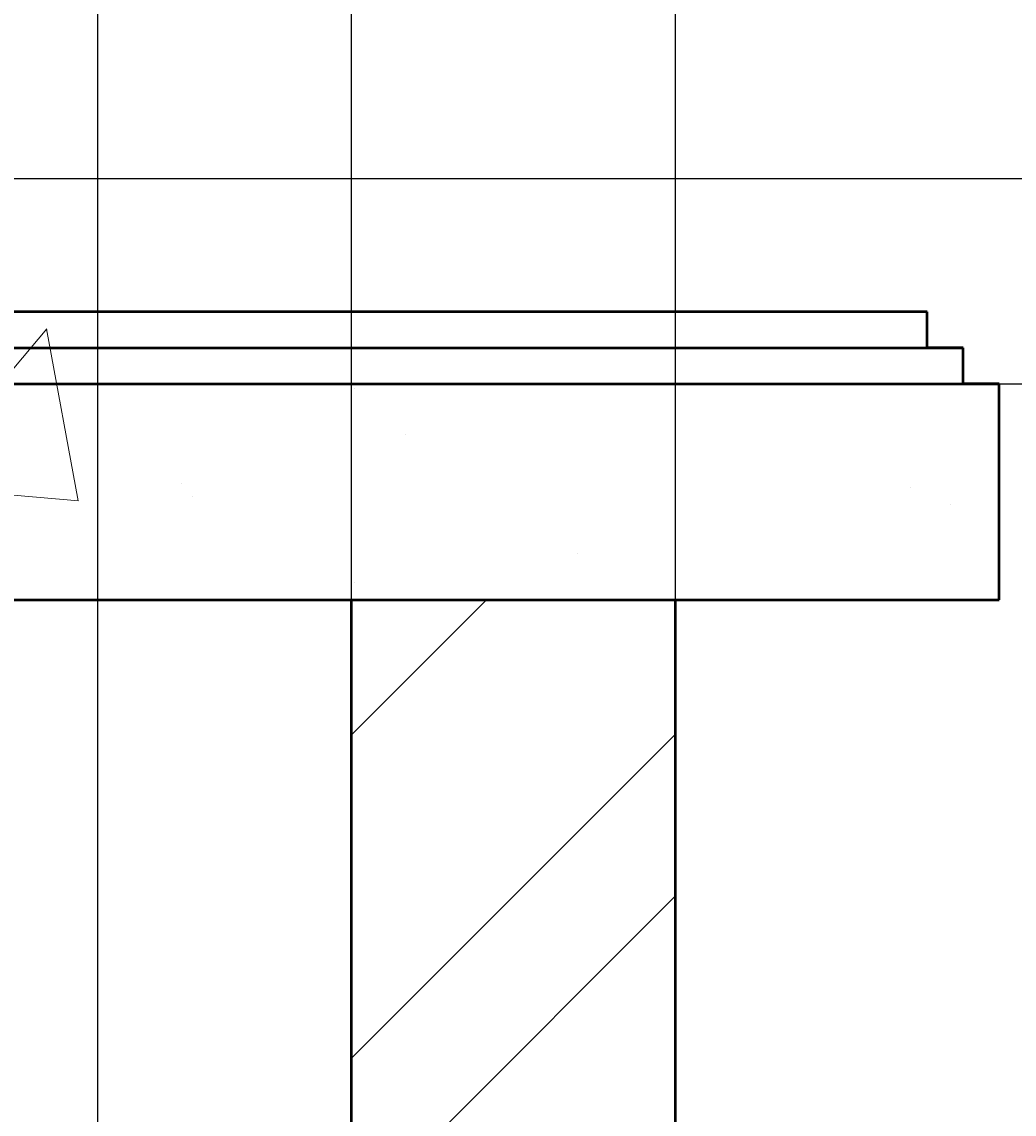
# Model space of a CAD drawing. Units: inches. Extents: x 2812 to 3051, y 1398 to 1659.
# Tile 41 of 65: x 3009 to 3037, y 1468 to 1498. Entities that reach past the tile are written whole.
import ezdxf

# ---------------------------------------------------------------- set-up
doc = ezdxf.new("R2010")
doc.units = ezdxf.units.IN
for name, color, linetype, lineweight in [('A-ANNO-DIMS', 2, 'Continuous', 18), ('S-CONC', 7, 'Continuous', 50), ('S-CONC-PATT', 8, 'Continuous', 18)]:
    doc.layers.add(name, color=color, linetype=linetype, lineweight=lineweight)
doc.styles.get("Standard").update_dxf_attribs({"font": 'arial.ttf'})
doc.dimstyles.get("Standard").update_dxf_attribs({"dimtxt": 0.18, "dimasz": 0.18, "dimexe": 0.18, "dimexo": 0.0625, "dimgap": 0.09, "dimtad": 0, "dimtih": 1, "dimtoh": 1, "dimdec": 4, "dimzin": 0, "dimdsep": 46, "dimtxsty": 'Standard', "dimcen": 0.09, "dimadec": 0, "dimazin": 0, "dimtfac": 1, "dimtdec": 4, "dimtofl": 0, "dimtmove": 0, "dimatfit": 3, "dimfxl": 1, "dimtolj": 1, "dimtzin": 0, "dimarcsym": 0})

# ---------------------------------------------------------------- blocks, each defined once
blk = doc.blocks.new('*D33')
at = {"layer": 'A-ANNO-DIMS', "color": 0, "lineweight": -2, "transparency": 16777216}
for p, q in [((3011.337, 1597.982), (3011.337, 1397.505)), ((3018.385, 1559.757), (3018.385, 1397.505)), ((3011.517, 1397.685), (3014.468, 1397.685)), ((3018.205, 1397.685), (3015.254, 1397.685))]:
    blk.add_line(p, q, dxfattribs=at)
at = {"layer": 'A-ANNO-DIMS', "color": 0, "transparency": 16777216}
for points in [[(3011.517, 1397.715), (3011.517, 1397.655), (3011.337, 1397.685)], [(3018.205, 1397.715), (3018.205, 1397.655), (3018.385, 1397.685)]]:
    blk.add_solid(points, dxfattribs=at)
at = {"layer": 'Defpoints', "color": 0, "transparency": 16777216}
for p in [(3011.337, 1598.044), (3018.385, 1559.82), (3018.385, 1397.685)]:
    blk.add_point(p, dxfattribs=at)
at = {"layer": 'A-ANNO-DIMS', "color": 0, "transparency": 16777216, "insert": (3014.861, 1397.685), "char_height": 0.18, "attachment_point": 5}
blk.add_mtext('\\A1;7.048', dxfattribs=at)
blk = doc.blocks.new('*D34')
at = {"layer": 'A-ANNO-DIMS', "color": 0, "lineweight": -2, "transparency": 16777216}
for p, q in [((3038.462, 1593.482), (3038.462, 1397.505)), ((3027.385, 1550.757), (3027.385, 1397.505)), ((3027.565, 1397.685), (3032.468, 1397.685)), ((3038.282, 1397.685), (3033.379, 1397.685))]:
    blk.add_line(p, q, dxfattribs=at)
at = {"layer": 'A-ANNO-DIMS', "color": 0, "transparency": 16777216}
for points in [[(3027.565, 1397.715), (3027.565, 1397.655), (3027.385, 1397.685)], [(3038.282, 1397.715), (3038.282, 1397.655), (3038.462, 1397.685)]]:
    blk.add_solid(points, dxfattribs=at)
at = {"layer": 'Defpoints', "color": 0, "transparency": 16777216}
for p in [(3038.462, 1593.544), (3027.385, 1550.82), (3038.462, 1397.685)]:
    blk.add_point(p, dxfattribs=at)
at = {"layer": 'A-ANNO-DIMS', "color": 0, "transparency": 16777216, "insert": (3032.923, 1397.685), "char_height": 0.18, "attachment_point": 5}
blk.add_mtext('\\A1;11.077', dxfattribs=at)
blk = doc.blocks.new('*D48')
at = {"layer": 'A-ANNO-DIMS', "color": 0, "lineweight": -2, "transparency": 16777216}
for p, q in [((3006.385, 1487.973), (3006.385, 1397.505)), ((3036.385, 1409.973), (3036.385, 1397.505)), ((3006.565, 1397.685), (3021.166, 1397.685)), ((3036.205, 1397.685), (3021.603, 1397.685))]:
    blk.add_line(p, q, dxfattribs=at)
at = {"layer": 'A-ANNO-DIMS', "color": 0, "transparency": 16777216}
for points in [[(3006.565, 1397.715), (3006.565, 1397.655), (3006.385, 1397.685)], [(3036.205, 1397.715), (3036.205, 1397.655), (3036.385, 1397.685)]]:
    blk.add_solid(points, dxfattribs=at)
at = {"layer": 'Defpoints', "color": 0, "transparency": 16777216}
for p in [(3006.385, 1488.035), (3036.385, 1410.035), (3036.385, 1397.685)]:
    blk.add_point(p, dxfattribs=at)
at = {"layer": 'A-ANNO-DIMS', "color": 0, "transparency": 16777216, "insert": (3021.385, 1397.685), "char_height": 0.18, "attachment_point": 5}
blk.add_mtext('\\A1;30', dxfattribs=at)
blk = doc.blocks.new('*D54')
at = {"layer": 'A-ANNO-DIMS', "color": 0, "lineweight": -2, "transparency": 16777216}
for p, q in [((3036.447, 1488.035), (3051.178, 1488.035)), ((3050.998, 1487.855), (3050.998, 1449.217)), ((3050.998, 1410.215), (3050.998, 1448.853)), ((3036.447, 1410.035), (3051.178, 1410.035))]:
    blk.add_line(p, q, dxfattribs=at)
at = {"layer": 'A-ANNO-DIMS', "color": 0, "transparency": 16777216}
for points in [[(3050.968, 1487.855), (3051.028, 1487.855), (3050.998, 1488.035)], [(3050.968, 1410.215), (3051.028, 1410.215), (3050.998, 1410.035)]]:
    blk.add_solid(points, dxfattribs=at)
at = {"layer": 'Defpoints', "color": 0, "transparency": 16777216}
for p in [(3036.385, 1488.035), (3050.998, 1488.035), (3036.385, 1410.035)]:
    blk.add_point(p, dxfattribs=at)
at = {"layer": 'A-ANNO-DIMS', "color": 0, "transparency": 16777216, "insert": (3050.998, 1449.035), "char_height": 0.18, "attachment_point": 5}
blk.add_mtext('\\A1;78', dxfattribs=at)
blk = doc.blocks.new('*D55')
at = {"layer": 'A-ANNO-DIMS', "color": 0, "lineweight": -2, "transparency": 16777216}
for p, q in [((2850.811, 1493.738), (3051.178, 1493.738)), ((3050.998, 1493.558), (3050.998, 1491.069)), ((3050.998, 1488.215), (3050.998, 1490.705)), ((2850.811, 1488.035), (3051.178, 1488.035))]:
    blk.add_line(p, q, dxfattribs=at)
at = {"layer": 'A-ANNO-DIMS', "color": 0, "transparency": 16777216}
for points in [[(3050.968, 1493.558), (3051.028, 1493.558), (3050.998, 1493.738)], [(3050.968, 1488.215), (3051.028, 1488.215), (3050.998, 1488.035)]]:
    blk.add_solid(points, dxfattribs=at)
at = {"layer": 'Defpoints', "color": 0, "transparency": 16777216}
for p in [(2850.748, 1493.738), (3050.998, 1493.738), (2850.748, 1488.035)]:
    blk.add_point(p, dxfattribs=at)
at = {"layer": 'A-ANNO-DIMS', "color": 0, "transparency": 16777216, "insert": (3050.998, 1490.887), "char_height": 0.18, "attachment_point": 5}
blk.add_mtext('\\A1;5.703', dxfattribs=at)

msp = doc.modelspace()

# ---------------------------------------------------------------- hatches: boundary and pattern name
at = {"layer": 'S-CONC-PATT'}
h = msp.add_hatch(dxfattribs=at)
h.set_pattern_fill('ANSI32', color=256)
h.paths.add_polyline_path([(3027.3849, 1646.82), (2835.3849, 1646.82), (2835.3849, 1603.2296), (2844.3849, 1603.2296), (2844.3849, 1637.82), (3018.3849, 1637.82), (3018.3849, 1602.5441), (3027.3849, 1602.5441)])
h.paths.add_polyline_path([(2844.3849, 1594.2296), (2835.3849, 1594.2296), (2835.3849, 1550.82), (3027.3849, 1550.82), (3027.3849, 1593.5441), (3018.3849, 1593.5441), (3018.3849, 1559.82), (2844.3849, 1559.82)])
h.paths.add_polyline_path([(2844.3849, 1482.0354), (2835.3849, 1482.0354), (2835.3849, 1463.4959), (2844.3849, 1463.4959)])
h.paths.add_polyline_path([(2844.3849, 1461.4959), (2835.3849, 1461.4959), (2835.3849, 1416.0354), (2844.3849, 1416.0354)])
h.paths.add_polyline_path([(3027.3849, 1482.0354), (3018.3849, 1482.0354), (3018.3849, 1463.2854), (3027.3849, 1463.2854)])
h.paths.add_polyline_path([(3027.3849, 1461.2854), (3018.3849, 1461.2854), (3018.3849, 1416.0354), (3027.3849, 1416.0354)])
h.paths.add_polyline_path([(2961.3849, 1448.4738), (2952.3849, 1448.4738), (2952.3849, 1416.0354), (2961.3849, 1416.0354)])
h.paths.add_polyline_path([(2961.3849, 1462.3026), (2952.3849, 1462.3026), (2952.3849, 1450.4738), (2961.3849, 1450.4738)])
h.paths.add_polyline_path([(2961.3849, 1472.0354), (2952.3849, 1472.0354), (2952.3849, 1462.3026), (2961.3849, 1462.3026)])
h = msp.add_hatch(dxfattribs=at)
h.set_pattern_fill('AR-SAND', color=256, scale=0.3)
h.paths.add_polyline_path([(3036.3849, 1416.0354), (3027.3849, 1416.0354), (2826.3849, 1416.0354), (2826.3849, 1410.0354), (2835.3849, 1410.0354), (3036.3849, 1410.0354)])
h.paths.add_polyline_path([(2970.3849, 1488.0354), (2969.3849, 1488.0354), (2941.3849, 1488.0354), (2941.3849, 1482.0354), (2970.3849, 1482.0354)])
h.paths.add_polyline_path([(3036.3849, 1488.0354), (3035.3849, 1488.0354), (3006.3849, 1488.0354), (3006.3849, 1482.0354), (3027.3849, 1482.0354), (3036.3849, 1482.0354)])
h.paths.add_polyline_path([(3034.3849, 1490.0354), (3008.3849, 1490.0354), (3008.3849, 1489.0354), (3034.3849, 1489.0354)])
h.paths.add_polyline_path([(3035.3849, 1489.0354), (3034.3849, 1489.0354), (3007.3849, 1489.0354), (3007.3849, 1488.0354), (3035.3849, 1488.0354)])
h.paths.add_polyline_path([(2968.3849, 1490.0354), (2943.3849, 1490.0354), (2943.3849, 1489.0354), (2968.3849, 1489.0354)])
h.paths.add_polyline_path([(2969.3849, 1489.0354), (2968.3849, 1489.0354), (2942.3849, 1489.0354), (2942.3849, 1488.0354), (2969.3849, 1488.0354)])
h.paths.add_polyline_path([(2896.3849, 1488.0354), (2826.3849, 1488.0354), (2826.3849, 1482.0354), (2896.3849, 1482.0354)])
h.paths.add_polyline_path([(2895.3849, 1489.0354), (2894.3849, 1489.0354), (2827.3849, 1489.0354), (2827.3849, 1488.0354), (2895.3849, 1488.0354)])
h.paths.add_polyline_path([(2894.3849, 1490.0354), (2828.3849, 1490.0354), (2828.3849, 1489.0354), (2894.3849, 1489.0354)])
h = msp.add_hatch(dxfattribs=at)
h.set_pattern_fill('AR-CONC', color=256, scale=0.3)
h.paths.add_polyline_path([(2896.3849, 1488.0354), (2826.3849, 1488.0354), (2826.3849, 1482.0354), (2896.3849, 1482.0354)])
h.paths.add_polyline_path([(2970.3849, 1488.0354), (2941.3849, 1488.0354), (2941.3849, 1482.0354), (2970.3849, 1482.0354)])
h.paths.add_polyline_path([(2968.3849, 1490.0354), (2943.3849, 1490.0354), (2943.3849, 1489.0354), (2968.3849, 1489.0354)])
h.paths.add_polyline_path([(2969.3849, 1489.0354), (2968.3849, 1489.0354), (2943.3849, 1489.0354), (2942.3849, 1489.0354), (2942.3849, 1488.0354), (2969.3849, 1488.0354)])
h.paths.add_polyline_path([(3036.3849, 1488.0354), (3035.3849, 1488.0354), (3006.3849, 1488.0354), (3006.3849, 1482.0354), (3027.3849, 1482.0354), (3036.3849, 1482.0354)])
h.paths.add_polyline_path([(3035.3849, 1489.0354), (3034.3849, 1489.0354), (3007.3849, 1489.0354), (3007.3849, 1488.0354), (3035.3849, 1488.0354)])
h.paths.add_polyline_path([(3034.3849, 1490.0354), (3008.3849, 1490.0354), (3008.3849, 1489.0354), (3034.3849, 1489.0354)])
h.paths.add_polyline_path([(2895.3849, 1489.0354), (2894.3849, 1489.0354), (2827.3849, 1489.0354), (2827.3849, 1488.0354), (2895.3849, 1488.0354)])
h.paths.add_polyline_path([(2894.3849, 1490.0354), (2828.3849, 1490.0354), (2828.3849, 1489.0354), (2894.3849, 1489.0354)])

# ---------------------------------------------------------------- linework, layer by layer
at = {"layer": 'S-CONC'}
for p, q in [((3034.3849, 1490.0354), (2850.7485, 1490.0354)), ((3034.3849, 1489.0354), (3034.3849, 1490.0354)), ((2850.7485, 1489.0354), (3035.3849, 1489.0354)), ((3035.3849, 1489.0354), (3034.3849, 1489.0354)), ((3035.3849, 1488.0354), (3035.3849, 1489.0354)), ((2850.7485, 1488.0354), (3036.3849, 1488.0354)), ((3036.3849, 1488.0354), (3035.3849, 1488.0354)), ((3036.3849, 1482.0354), (3036.3849, 1488.0354)), ((2850.7485, 1482.0354), (3027.3849, 1482.0354)), ((3018.3849, 1482.0354), (3018.3849, 1416.0354)), ((3027.3849, 1482.0354), (3027.3849, 1416.0354)), ((3027.3849, 1482.0354), (3036.3849, 1482.0354))]:
    msp.add_line(p, q, dxfattribs=at)

# ---------------------------------------------------------------- dimensions: what is measured, and where the dimension line sits
at = {"layer": 'A-ANNO-DIMS'}
for base, p1, p2, override, picture, middle in [((3018.3849, 1397.6854), (3011.3373, 1598.0441), (3018.3849, 1559.82), {"dimdec": 3, "dimlfac": 1, "dimrnd": 0, "dimzin": 0, "dimdsep": 46, "dimlunit": 2}, '*D33', (3014.8611, 1397.6854)), ((3038.4621, 1397.6854), (3027.3849, 1550.82), (3038.4621, 1593.5441), {"dimdec": 3, "dimlfac": 1, "dimrnd": 0, "dimzin": 0, "dimdsep": 46, "dimlunit": 2}, '*D34', (3032.9235, 1397.6854)), ((3036.3849, 1397.6854), (3006.3849, 1488.0354), (3036.3849, 1410.0354), {"dimdec": 0, "dimlfac": 1, "dimrnd": 0, "dimzin": 0, "dimdsep": 46, "dimlunit": 2}, '*D48', (3021.3849, 1397.6854))]:
    dim = msp.add_linear_dim(base=base, p1=p1, p2=p2, dimstyle='Standard', override=override, dxfattribs=at)
    dim.commit()
    dim.dimension.update_dxf_attribs({"geometry": picture, "text_midpoint": middle})
for base, p1, p2, override, picture, middle in [((3050.998, 1493.7383), (2850.7485, 1488.0354), (2850.7485, 1493.7383), {"dimdec": 3, "dimlfac": 1, "dimrnd": 0, "dimzin": 0, "dimdsep": 46, "dimlunit": 2}, '*D55', (3050.998, 1490.8868)), ((3050.998, 1488.0354), (3036.3849, 1410.0354), (3036.3849, 1488.0354), {"dimdec": 0, "dimlfac": 1, "dimrnd": 0, "dimzin": 0, "dimdsep": 46, "dimlunit": 2}, '*D54', (3050.998, 1449.0354))]:
    dim = msp.add_linear_dim(base=base, p1=p1, p2=p2, angle=90, dimstyle='Standard', override=override, dxfattribs=at)
    dim.commit()
    dim.dimension.update_dxf_attribs({"geometry": picture, "text_midpoint": middle})

doc.saveas('drawing.dxf')
